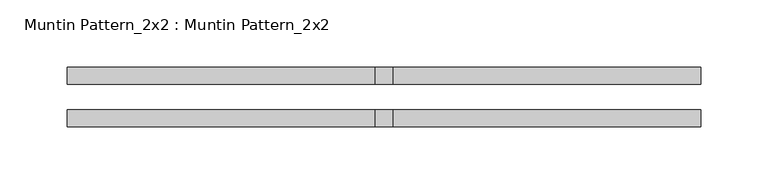
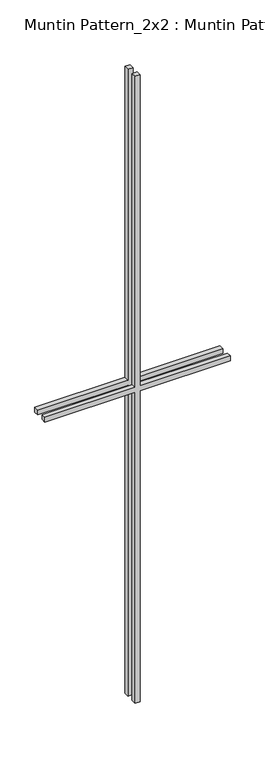
"""IFC4 building model written with IfcOpenShell, lengths in millimetres: proxy geometry, Muntin Pattern_2x2 : Muntin Pattern_2x2."""

from ifc_helpers import new_model, si_unit, frame, origin, place, context, project, spatial, polyline, outline, extrude, source, transform, mapped, element, save


def muntin_pattern_2x2_muntin_pattern_2x2_2b4d9f72(model_context):
    return source(origin(), model_context, "Body", "SweptSolid", [
        extrude(outline(polyline([(850.9, -6.35), (850.9, -236.5375), (838.2, -236.5375), (838.2, -6.35), (0.0, -6.35), (0.0, 6.35), (838.2, 6.35), (838.2, 236.5375), (850.9, 236.5375), (850.9, 6.35), (1689.1, 6.35), (1689.1, -6.35), (850.9, -6.35)])), frame((0.0, 9.525, 0.0), z_axis=(0.0, 1.0, 0.0), x_axis=(0.0, 0.0, 1.0)), (0.0, 0.0, 1.0), 12.7),
        extrude(outline(polyline([(850.9, -6.35), (850.9, -236.5375), (838.2, -236.5375), (838.2, -6.35), (0.0, -6.35), (0.0, 6.35), (838.2, 6.35), (838.2, 236.5375), (850.9, 236.5375), (850.9, 6.35), (1689.1, 6.35), (1689.1, -6.35), (850.9, -6.35)])), frame((0.0, -22.225, 0.0), z_axis=(0.0, 1.0, 0.0), x_axis=(0.0, 0.0, 1.0)), (0.0, 0.0, 1.0), 12.7),
    ])


if __name__ == "__main__":
    model = new_model("IFC4")
    model_context = context("Model", 3, world=origin())
    ifc_project = project(units=[si_unit("LENGTHUNIT", "METRE", prefix="MILLI")], contexts=[model_context])
    site = spatial("IfcSite", under=ifc_project)
    building = spatial("IfcBuilding", under=site)
    placement = place(None, origin())
    muntin_pattern_2x2_muntin_pattern_2x2_shape = muntin_pattern_2x2_muntin_pattern_2x2_2b4d9f72(model_context)
    element("IfcBuildingElementProxy", 1, Name="Muntin Pattern_2x2 : Muntin Pattern_2x2", ObjectType="Muntin Pattern_2x2 : Muntin Pattern_2x2", at=placement, inside=building, context=model_context, shape_type="MappedRepresentation", body=[
        mapped(muntin_pattern_2x2_muntin_pattern_2x2_shape, transform((0.0, 0.0, 0.0), x_axis=(1.0, 0.0, 0.0), y_axis=(0.0, 1.0, 0.0), z_axis=(0.0, 0.0, 1.0))),
    ])
    save(model, "model.ifc")

# Revit data of these elements
# Type "Muntin Pattern_2x2 : Muntin Pattern_2x2"
#   Width [instance default] = 4' - 0"
#   Thickness = 0' - 0 1/2"
#   Height [instance default] = 4' - 0"
#   Distance = 0' - 0 3/4"
#   Interior Material [instance default] = none
#   Exterior Material [instance default] = none
#   Default Elevation = 0
# Element 1 (IfcBuildingElementProxy, "Muntin Pattern_2x2 : Muntin Pattern_2x2")
#   Width = 1' - 6 5/8"
#   Height = 5' - 6 1/2"
#   Interior Material = Wood - Stained
#   Exterior Material = Clad - White
#   Materials on its faces: "Clad - White", "Wood - Stained"
# Materials
#   "Clad - White": class "Wood", colour RGB 242 242 238, transparency 0, Cost = 0
#   "Wood - Stained": class "Wood", colour RGB 224 178 126, transparency 0, Cost = 0
